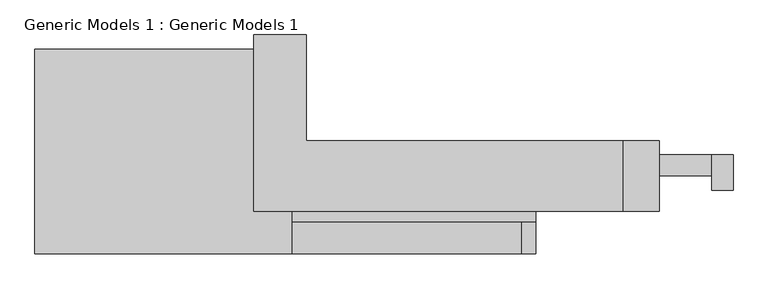
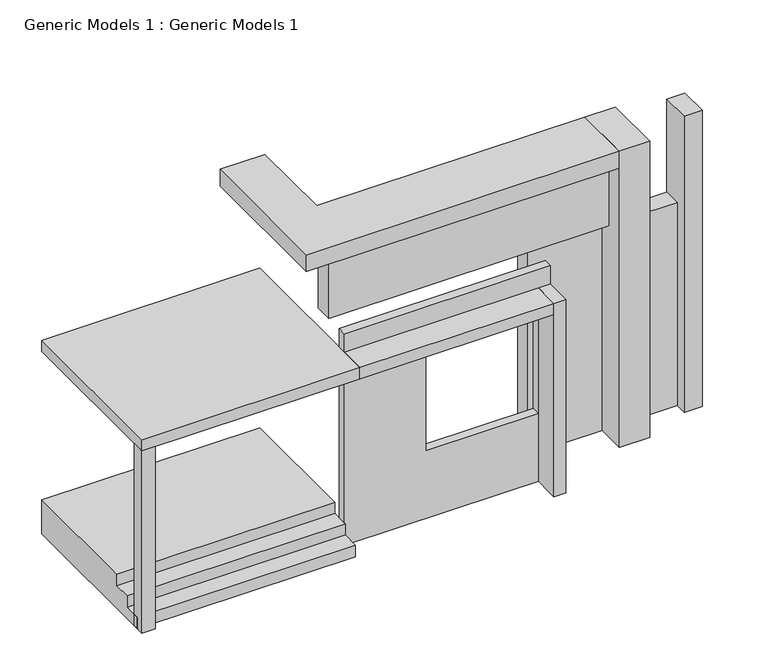
"""IFC4 building model written with IfcOpenShell, lengths in millimetres: proxy geometry, Generic Models 1 : Generic Models 1."""

from ifc_helpers import new_model, si_unit, frame, origin, origin_with_axes, place, context, project, spatial, polyline, outline, extrude, source, transform, mapped, element, save


def generic_models_1_generic_models_1_adbbf048(model_context):
    return source(origin(), model_context, "Body", "SweptSolid", [
        extrude(outline(polyline([(1106.440599, 5440.2433441), (344.440599, 5440.2433441), (344.440599, 5745.0433441), (1106.440599, 5745.0433441), (1106.440599, 5440.2433441)])), origin_with_axes(), (0.0, 0.0, 1.0), 3657.6),
        extrude(outline(polyline([(1411.240599, 5237.0433441), (1106.440599, 5237.0433441), (1106.440599, 5745.0433441), (1411.240599, 5745.0433441), (1411.240599, 5237.0433441)])), origin_with_axes(), (0.0, 0.0, 1.0), 5334.0),
        extrude(outline(polyline([(-170.9014886, 5440.2433441), (-1433.559401, 5440.2433441), (-1433.559401, 5745.0433441), (-170.9014886, 5745.0433441), (-170.9014886, 5440.2433441)])), origin_with_axes(), (0.0, 0.0, 1.0), 3810.0),
        extrude(outline(polyline([(-170.9014886, 5237.0433441), (-4938.759401, 5237.0433441), (-4938.759401, 5541.8433441), (-170.9014886, 5541.8433441), (-170.9014886, 5237.0433441)])), frame((0.0, 0.0, 3810.0), z_axis=(0.0, 0.0, 1.0), x_axis=(1.0, 0.0, 0.0)), (0.0, 0.0, 1.0), 1219.2),
        extrude(outline(polyline([(0.0, -4938.759401), (0.0, -1433.559401), (3810.0, -1433.559401), (3810.0, -4938.759401), (0.0, -4938.759401)]), holes=[polyline([(3073.4, -3541.759401), (3073.4, -1636.759401), (1219.2, -1636.759401), (1219.2, -3541.759401), (3073.4, -3541.759401)])]), frame((0.0, 4779.8433441, 0.0), z_axis=(0.0, 1.0, 0.0), x_axis=(0.0, 0.0, 1.0)), (0.0, 0.0, 1.0), 152.4),
        extrude(outline(polyline([(344.440599, 5948.2433441), (344.440599, 4932.2433441), (-170.9014886, 4932.2433441), (-170.9014886, 5948.2433441), (344.440599, 5948.2433441)])), origin_with_axes(), (0.0, 0.0, 1.0), 5334.0),
        extrude(outline(polyline([(-5497.559401, 7472.2433441), (-4735.559401, 7472.2433441), (-4735.559401, 5948.2433441), (-170.9014886, 5948.2433441), (-170.9014886, 4932.2433441), (-5497.559401, 4932.2433441), (-5497.559401, 7472.2433441)])), frame((0.0, 0.0, 5029.2), z_axis=(0.0, 0.0, 1.0), x_axis=(1.0, 0.0, 0.0)), (0.0, 0.0, 1.0), 304.8),
        extrude(outline(polyline([(-8418.559401, 4322.6433441), (-8647.159401, 4322.6433441), (-8647.159401, 4551.2433441), (-8418.559401, 4551.2433441), (-8418.559401, 4322.6433441)])), origin_with_axes(), (0.0, 0.0, 1.0), 3276.6),
        extrude(outline(polyline([(-1433.559401, 4322.6433441), (-1636.759401, 4322.6433441), (-1636.759401, 4932.2433441), (-1433.559401, 4932.2433441), (-1433.559401, 4322.6433441)])), origin_with_axes(), (0.0, 0.0, 1.0), 3479.8),
        extrude(outline(polyline([(-1636.759401, 4322.6433441), (-4938.759401, 4322.6433441), (-4938.759401, 4932.2433441), (-1636.759401, 4932.2433441), (-1636.759401, 4322.6433441)])), frame((0.0, 0.0, 3276.6), z_axis=(0.0, 0.0, 1.0), x_axis=(1.0, 0.0, 0.0)), (0.0, 0.0, 1.0), 203.2),
        extrude(outline(polyline([(-4938.759401, 4322.6433441), (-8647.159401, 4322.6433441), (-8647.159401, 7269.0433441), (-4938.759401, 7269.0433441), (-4938.759401, 4322.6433441)])), frame((0.0, 0.0, 3276.6), z_axis=(0.0, 0.0, 1.0), x_axis=(1.0, 0.0, 0.0)), (0.0, 0.0, 1.0), 203.2),
        extrude(outline(polyline([(7269.0433441, 609.6), (7269.0433441, 0.0), (4449.6433441, 0.0), (4449.6433441, 203.2), (4754.4433441, 203.2), (4754.4433441, 406.4), (5059.2433441, 406.4), (5059.2433441, 609.6), (7269.0433441, 609.6)])), frame((-8647.159401, 0.0, 0.0), z_axis=(1.0, 0.0, 0.0), x_axis=(0.0, 1.0, 0.0)), (0.0, 0.0, 1.0), 3708.4),
    ])


if __name__ == "__main__":
    model = new_model("IFC4")
    model_context = context("Model", 3, world=origin())
    ifc_project = project(units=[si_unit("LENGTHUNIT", "METRE", prefix="MILLI")], contexts=[model_context])
    site = spatial("IfcSite", under=ifc_project)
    building = spatial("IfcBuilding", under=site)
    placement = place(None, origin())
    generic_models_1_generic_models_1_shape = generic_models_1_generic_models_1_adbbf048(model_context)
    element("IfcBuildingElementProxy", 1, Name="Generic Models 1 : Generic Models 1", ObjectType="Generic Models 1 : Generic Models 1", at=placement, inside=building, context=model_context, shape_type="MappedRepresentation", body=[
        mapped(generic_models_1_generic_models_1_shape, transform((0.0, 0.0, 0.0), x_axis=(1.0, 0.0, 0.0), y_axis=(0.0, 1.0, 0.0), z_axis=(0.0, 0.0, 1.0))),
    ])
    save(model, "model.ifc")
